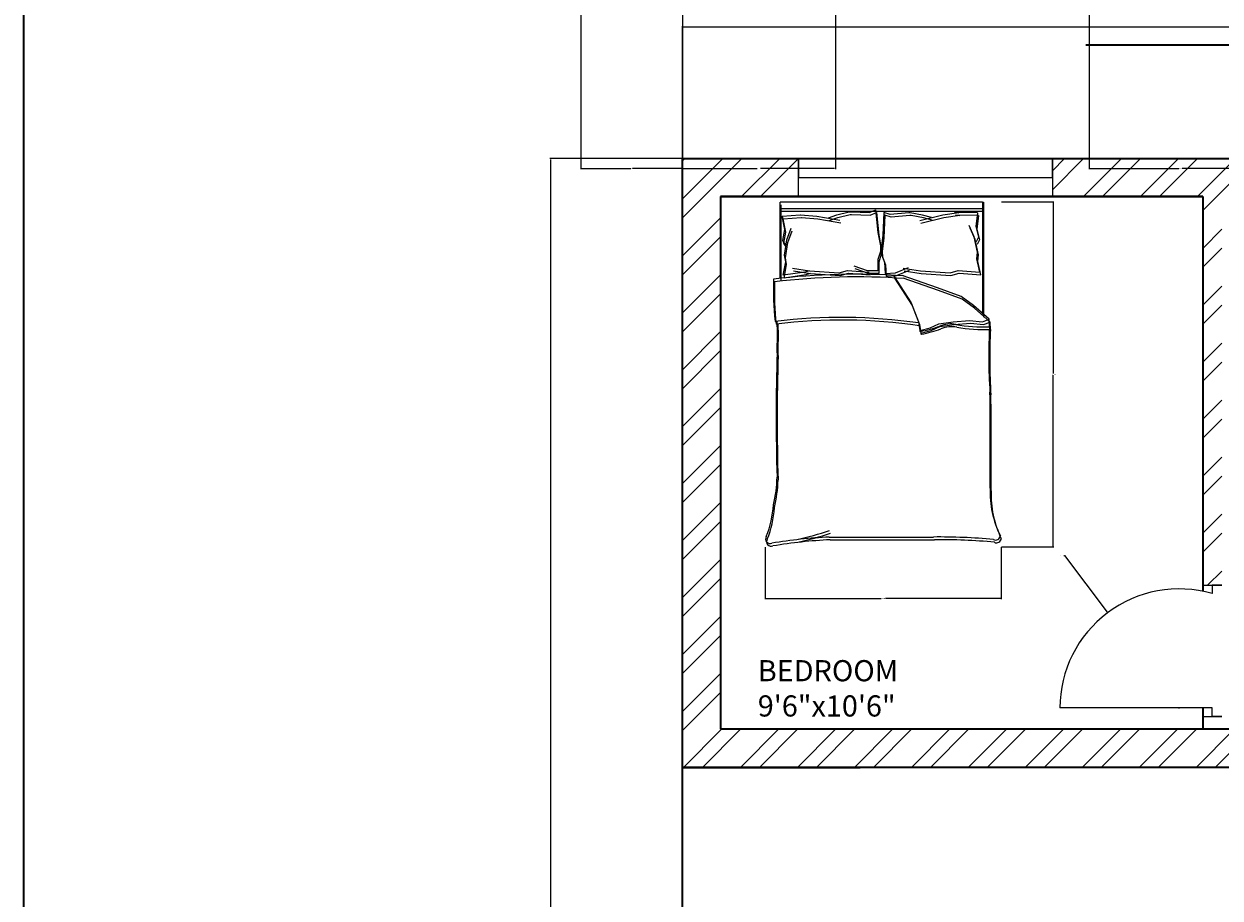
# Model space of a CAD drawing. Units: inches. Extents: x 1955 to 3324, y 980 to 3129.
# Tile 4 of 11: x 1955 to 2237, y 2282 to 2488. Entities that reach past the tile are written whole.
import ezdxf

# ---------------------------------------------------------------- set-up
doc = ezdxf.new("R2010")
doc.units = ezdxf.units.IN
for name, color, linetype, lineweight in [('A-ANNO-DIMS', 2, 'Continuous', 18), ('A-ANNO-TITL', 7, 'Continuous', 35), ('A-ANNO-TTLB', 7, 'Continuous', 35), ('A-AREA-IDEN', 7, 'Continuous', 18), ('A-DOOR', 3, 'Continuous', 18), ('A-FURN', 8, 'Continuous', 18), ('A-GLAZ', 4, 'Continuous', 18), ('A-WALL', 7, 'Continuous', 35), ('A-WALL-PATT', 252, 'Continuous', 13)]:
    doc.layers.add(name, color=color, linetype=linetype, lineweight=lineweight)
doc.styles.get("Standard").update_dxf_attribs({"font": 'arial.ttf'})
doc.dimstyles.get("Standard").update_dxf_attribs({"dimtxt": 0.18, "dimasz": 0.18, "dimexe": 0.18, "dimexo": 0.0625, "dimgap": 0.09, "dimtad": 0, "dimtih": 1, "dimtoh": 1, "dimdec": 4, "dimzin": 0, "dimdsep": 46, "dimtxsty": 'Standard', "dimcen": 0.09, "dimadec": 0, "dimazin": 0, "dimtfac": 1, "dimtdec": 4, "dimtofl": 0, "dimtmove": 0, "dimatfit": 3, "dimfxl": 1, "dimtolj": 1, "dimtzin": 0, "dimarcsym": 0})

# ---------------------------------------------------------------- blocks, each defined once
blk = doc.blocks.new('BED-WITH-PILLOWS')
for p, q in [((3.48, 63.33), (3.48, 81.44)), ((3.48, 63.33), (3.48, 81.44)), ((51.27, 81.44), (3.48, 81.44)), ((3.48, 79.91), (51.27, 79.91)), ((3.48, 79.91), (51.27, 79.91)), ((3.7, 62.69), (3.7, 80.8)), ((3.7, 62.69), (3.7, 80.8)), ((3.7, 79.27), (51.49, 79.27)), ((3.7, 79.27), (51.49, 79.27)), ((24.54, 78.99), (25.98, 79.57)), ((24.54, 78.99), (25.98, 79.57)), ((25.98, 79.57), (26.56, 74.22)), ((25.98, 79.57), (26.56, 74.22)), ((51.27, 81.44), (51.27, 54.83)), ((51.27, 81.44), (51.27, 54.83)), ((51.27, 81.44), (51.49, 81.44)), ((51.49, 81.44), (51.49, 80.8)), ((51.49, 80.8), (51.49, 54.19)), ((51.49, 80.8), (51.49, 54.19)), ((3.89, 78.13), (4.47, 74.95)), ((3.9, 78.11), (8.18, 78.43)), ((3.9, 78.11), (8.18, 78.43)), ((3.9, 78.13), (4.47, 74.95)), ((4.12, 77.49), (4.7, 74.31)), ((4.12, 77.49), (4.7, 74.31)), ((4.13, 77.47), (8.41, 77.8)), ((4.13, 77.47), (8.41, 77.8)), ((8.18, 78.43), (8.29, 78.42)), ((8.18, 78.43), (8.29, 78.42)), ((8.29, 78.42), (12.11, 78.13)), ((8.29, 78.42), (12.11, 78.13)), ((8.41, 77.8), (8.51, 77.78)), ((8.41, 77.8), (8.51, 77.78)), ((8.51, 77.78), (12.34, 77.49)), ((8.51, 77.78), (12.34, 77.49)), ((12.11, 78.13), (17.6, 77.12)), ((12.11, 78.13), (17.6, 77.12)), ((12.34, 77.49), (17.83, 76.48)), ((12.34, 77.49), (17.83, 76.48)), ((14.86, 77.69), (16.88, 78.42)), ((14.86, 77.69), (16.88, 78.42)), ((15.08, 77.05), (17.11, 77.78)), ((15.08, 77.05), (17.11, 77.78)), ((16.88, 78.42), (19.77, 79.14)), ((16.88, 78.42), (19.77, 79.14)), ((17.11, 77.78), (20, 78.5)), ((17.11, 77.78), (20, 78.5)), ((19.77, 79.14), (20.09, 79.14)), ((19.77, 79.14), (20.09, 79.14)), ((20, 78.5), (20.32, 78.5)), ((20, 78.5), (20.32, 78.5)), ((20.09, 79.14), (24.54, 78.99)), ((20.09, 79.14), (24.54, 78.99)), ((20.32, 78.5), (24.77, 78.36)), ((20.32, 78.5), (24.77, 78.36)), ((24.77, 78.36), (26.21, 78.93)), ((24.77, 78.36), (26.21, 78.93)), ((26.21, 78.93), (26.79, 73.58)), ((26.21, 78.93), (26.79, 73.58)), ((27.98, 78.95), (27.73, 73.58)), ((27.98, 78.95), (27.73, 73.58)), ((28.21, 78.31), (27.96, 72.94)), ((28.21, 78.31), (27.96, 72.94)), ((29.46, 78.46), (27.98, 78.95)), ((29.46, 78.46), (27.98, 78.95)), ((29.68, 77.83), (28.21, 78.31)), ((29.68, 77.83), (28.21, 78.31)), ((33.88, 78.89), (29.46, 78.46)), ((33.88, 78.89), (29.46, 78.46)), ((34.11, 78.25), (29.68, 77.83)), ((34.11, 78.25), (29.68, 77.83)), ((34.21, 78.91), (33.88, 78.89)), ((34.2, 78.91), (33.88, 78.89)), ((34.43, 78.27), (34.11, 78.25)), ((34.43, 78.27), (34.11, 78.25)), ((37.14, 78.36), (34.2, 78.91)), ((37.14, 78.36), (34.21, 78.91)), ((37.36, 77.73), (34.43, 78.27)), ((37.36, 77.73), (34.43, 78.27)), ((41.91, 78.37), (36.5, 77.02)), ((41.91, 78.37), (36.5, 77.02)), ((42.14, 77.73), (36.72, 76.38)), ((42.14, 77.73), (36.72, 76.38)), ((39.2, 77.77), (37.14, 78.36)), ((39.2, 77.77), (37.14, 78.36)), ((39.43, 77.13), (37.36, 77.73)), ((39.43, 77.13), (37.36, 77.73)), ((45.71, 78.9), (41.91, 78.37)), ((45.71, 78.9), (41.91, 78.37)), ((45.94, 78.26), (42.14, 77.73)), ((45.94, 78.26), (42.14, 77.73)), ((50.11, 78.89), (44.71, 78.98)), ((44.71, 78.98), (45.71, 78.9)), ((50.11, 78.89), (44.71, 78.98)), ((44.71, 78.98), (45.71, 78.9)), ((50.34, 78.25), (44.94, 78.34)), ((44.94, 78.34), (45.94, 78.26)), ((50.34, 78.25), (44.94, 78.34)), ((44.94, 78.34), (45.94, 78.26)), ((50.11, 78.89), (49.73, 75.68)), ((50.11, 78.89), (49.73, 75.68)), ((50.34, 78.25), (49.96, 75.04)), ((50.34, 78.25), (49.96, 75.04)), ((4.47, 74.95), (4.04, 72.34)), ((4.47, 74.95), (4.04, 72.34)), ((4.7, 74.31), (4.27, 71.7)), ((4.7, 74.31), (4.27, 71.7)), ((5.05, 72.49), (6.06, 75.24)), ((5.05, 72.49), (6.06, 75.24)), ((5.28, 71.85), (6.29, 74.6)), ((5.28, 71.85), (6.29, 74.6)), ((26.56, 74.22), (27.14, 71.04)), ((26.56, 74.22), (27.14, 71.04)), ((26.79, 73.58), (27.37, 70.4)), ((26.79, 73.58), (27.37, 70.4)), ((27.73, 73.58), (27.36, 70.37)), ((27.73, 73.58), (27.36, 70.37)), ((49.31, 73.19), (48.13, 75.86)), ((49.31, 73.19), (48.13, 75.86)), ((49.54, 72.55), (48.36, 75.23)), ((49.54, 72.55), (48.36, 75.23)), ((49.73, 75.68), (50.33, 73.11)), ((49.73, 75.68), (50.33, 73.11)), ((49.96, 75.04), (50.56, 72.47)), ((49.96, 75.04), (50.56, 72.47)), ((4.04, 72.34), (4.62, 71.33)), ((4.04, 72.34), (4.62, 71.33)), ((4.27, 71.7), (4.85, 70.69)), ((4.27, 71.7), (4.85, 70.69)), ((4.47, 68.87), (5.05, 72.49)), ((4.47, 68.87), (5.05, 72.49)), ((4.7, 68.23), (5.28, 71.85)), ((4.7, 68.23), (5.28, 71.85)), ((27.14, 71.04), (27.14, 69.74)), ((27.14, 71.04), (27.14, 69.74)), ((27.96, 72.94), (27.58, 69.73)), ((27.96, 72.94), (27.58, 69.73)), ((50.11, 69.61), (49.31, 73.19)), ((50.11, 69.61), (49.31, 73.19)), ((50.34, 68.98), (49.54, 72.55)), ((50.34, 68.98), (49.54, 72.55)), ((50.33, 73.11), (49.81, 72.06)), ((50.33, 73.11), (49.82, 72.06)), ((50.56, 72.47), (50.04, 71.42)), ((50.56, 72.47), (50.04, 71.42)), ((4.76, 67.28), (4.47, 68.87)), ((4.76, 67.28), (4.47, 68.87)), ((4.99, 66.64), (4.7, 68.23)), ((4.99, 66.64), (4.7, 68.23)), ((27.14, 69.74), (26.56, 67.86)), ((27.14, 69.74), (26.56, 67.86)), ((27.37, 69.1), (26.79, 67.22)), ((27.37, 69.1), (26.79, 67.22)), ((27.36, 70.37), (27.44, 69.07)), ((27.36, 70.37), (27.44, 69.07)), ((27.37, 70.4), (27.37, 69.1)), ((27.37, 70.4), (27.37, 69.1)), ((27.44, 69.07), (28.13, 67.23)), ((27.44, 69.07), (28.13, 67.23)), ((27.58, 69.73), (27.66, 68.43)), ((27.58, 69.73), (27.66, 68.43)), ((27.66, 68.43), (28.36, 66.59)), ((27.66, 68.43), (28.36, 66.59)), ((49.92, 68.01), (50.11, 69.61)), ((49.92, 68.01), (50.11, 69.61)), ((50.7, 64.87), (49.92, 68.01)), ((50.7, 64.87), (49.92, 68.01)), ((50.15, 67.37), (50.34, 68.98)), ((50.15, 67.37), (50.34, 68.98)), ((4.18, 64.1), (4.76, 67.28)), ((4.18, 64.1), (4.76, 67.28)), ((4.41, 63.46), (4.99, 66.64)), ((4.41, 63.46), (4.99, 66.64)), ((6.38, 65.81), (10.41, 65.15)), ((6.38, 65.81), (10.41, 65.15)), ((6.61, 65.18), (10.64, 64.51)), ((6.61, 65.18), (10.64, 64.51)), ((10.41, 65.15), (9.28, 64.83)), ((10.41, 65.15), (9.28, 64.83)), ((10.41, 65.15), (17.42, 64.72)), ((10.41, 65.15), (17.42, 64.72)), ((17.42, 64.72), (19.38, 65.27)), ((17.42, 64.72), (19.38, 65.27)), ((19.38, 65.27), (24.52, 64.87)), ((19.38, 65.27), (24.52, 64.87)), ((24.1, 65.18), (20.96, 66.27)), ((24.1, 65.18), (20.96, 66.27)), ((24.33, 64.54), (21.19, 65.63)), ((24.33, 64.54), (21.19, 65.63)), ((26.56, 65.18), (24.1, 65.18)), ((26.56, 65.18), (24.1, 65.18)), ((26.56, 67.86), (26.56, 65.18)), ((26.56, 67.86), (26.56, 65.18)), ((26.79, 67.22), (26.79, 64.54)), ((26.79, 67.22), (26.79, 64.54)), ((28.13, 67.23), (28.3, 64.55)), ((28.13, 67.23), (28.3, 64.55)), ((28.36, 66.59), (28.53, 63.91)), ((28.36, 66.59), (28.53, 63.91)), ((30.75, 64.7), (33.82, 65.99)), ((30.75, 64.7), (33.82, 65.99)), ((30.98, 64.06), (34.05, 65.35)), ((30.98, 64.06), (34.05, 65.35)), ((32.56, 65.81), (36.6, 65.15)), ((32.56, 65.81), (36.6, 65.15)), ((32.79, 65.18), (36.83, 64.51)), ((32.79, 65.18), (36.82, 64.51)), ((36.6, 65.15), (43.61, 64.72)), ((36.6, 65.15), (43.61, 64.72)), ((43.61, 64.72), (45.57, 65.27)), ((43.61, 64.72), (45.57, 65.27)), ((45.57, 65.27), (50.7, 64.87)), ((45.57, 65.27), (50.7, 64.87)), ((50.93, 64.23), (50.15, 67.37)), ((50.93, 64.23), (50.15, 67.37)), ((9.28, 64.83), (4.18, 64.1)), ((9.28, 64.83), (4.18, 64.1)), ((9.51, 64.19), (4.41, 63.46)), ((9.51, 64.19), (4.41, 63.46)), ((10.64, 64.51), (9.51, 64.19)), ((10.64, 64.51), (9.51, 64.19)), ((10.64, 64.51), (17.65, 64.08)), ((10.64, 64.51), (17.65, 64.08)), ((17.65, 64.08), (19.61, 64.63)), ((17.65, 64.08), (19.61, 64.63)), ((19.61, 64.63), (24.74, 64.23)), ((19.61, 64.63), (24.74, 64.23)), ((26.79, 64.54), (24.33, 64.54)), ((26.79, 64.54), (24.33, 64.54)), ((28.3, 64.55), (30.75, 64.7)), ((28.3, 64.55), (30.75, 64.7)), ((28.53, 63.91), (30.98, 64.06)), ((28.53, 63.91), (30.98, 64.06)), ((30.26, 64.06), (34.45, 57.57)), ((30.26, 64.06), (34.45, 57.57)), ((30.49, 63.42), (34.68, 56.93)), ((30.49, 63.42), (34.68, 56.93)), ((40.64, 61.13), (32.31, 64.06)), ((40.64, 61.13), (32.31, 64.06)), ((40.87, 60.49), (32.53, 63.42)), ((40.87, 60.49), (32.54, 63.42)), ((36.82, 64.51), (43.83, 64.08)), ((36.83, 64.51), (43.84, 64.08)), ((43.83, 64.08), (45.8, 64.63)), ((43.84, 64.08), (45.8, 64.63)), ((45.8, 64.63), (50.93, 64.23)), ((45.8, 64.63), (50.93, 64.23)), ((46.22, 59.11), (40.64, 61.13)), ((46.22, 59.11), (40.64, 61.13)), ((46.45, 58.48), (40.87, 60.49)), ((46.45, 58.48), (40.87, 60.49)), ((34.45, 57.57), (36.15, 53.08)), ((34.45, 57.57), (36.15, 53.08)), ((34.68, 56.93), (36.38, 52.44)), ((34.68, 56.93), (36.38, 52.44)), ((49.16, 56.95), (46.22, 59.11)), ((49.16, 56.95), (46.22, 59.11)), ((49.39, 56.31), (46.45, 58.48)), ((49.39, 56.31), (46.45, 58.48)), ((52.87, 53.7), (49.16, 56.95)), ((52.87, 53.7), (49.16, 56.95)), ((53.1, 53.06), (49.39, 56.31)), ((53.1, 53.06), (49.39, 56.31)), ((36.15, 53.08), (36.46, 51.07)), ((36.15, 53.08), (36.46, 51.07)), ((36.38, 52.44), (36.69, 50.43)), ((36.38, 52.44), (36.69, 50.43)), ((36.46, 51.07), (38.94, 51.69)), ((36.46, 51.07), (38.94, 51.69)), ((36.69, 50.43), (39.17, 51.05)), ((36.69, 50.43), (39.17, 51.05)), ((38.94, 51.69), (40.95, 52.61)), ((38.94, 51.69), (40.95, 52.61)), ((39.17, 51.05), (41.18, 51.97)), ((39.17, 51.05), (41.18, 51.97)), ((40.95, 52.61), (44.36, 53.08)), ((40.95, 52.61), (44.36, 53.08)), ((41.18, 51.97), (44.59, 52.44)), ((41.18, 51.97), (44.59, 52.44)), ((44.36, 53.08), (48.23, 53.39)), ((44.36, 53.08), (48.23, 53.39)), ((44.59, 52.44), (48.46, 52.75)), ((44.59, 52.44), (48.46, 52.75)), ((48.23, 53.39), (51.33, 53.08)), ((48.23, 53.39), (51.33, 53.08)), ((48.46, 52.75), (51.56, 52.44)), ((48.46, 52.75), (51.56, 52.44)), ((51.33, 53.08), (52.87, 53.7)), ((51.33, 53.08), (52.87, 53.7)), ((51.56, 52.44), (53.1, 53.06)), ((51.56, 52.44), (53.1, 53.06)), ((52.95, 51.95), (52.87, 53.7, 3.87)), ((52.95, 51.95), (52.87, 53.7, 3.87)), ((53.18, 51.31), (53.1, 53.06, 3.87)), ((53.18, 51.31), (53.1, 53.06, 3.87)), ((15.06, 2.2), (39.68, 2.2)), ((15.06, 2.2), (39.68, 2.2)), ((15.29, 1.56), (39.91, 1.56)), ((15.29, 1.56), (39.91, 1.56))]:
    blk.add_line(p, q)
for centre, radius, start, end in [((85.16, 61.35), 83.31, 178.7218, 185.604), ((85.16, 61.35), 83.31, 178.7218, 185.604), ((21.36, -100.61), 164.97, 86.0865, 96.7821), ((21.36, -100.61), 164.97, 86.0865, 96.7821), ((85.39, 60.71), 83.31, 178.7218, 185.604), ((85.39, 60.71), 83.31, 178.7218, 185.604), ((21.59, -101.25), 164.97, 86.0865, 96.7821), ((21.59, -101.25), 164.97, 86.0865, 96.7821), ((17.76, -74.87), 129.02, 81.7845, 96.9006), ((17.76, -74.87), 129.02, 81.7845, 96.9006), ((17.98, -75.51), 129.02, 81.7845, 96.9006), ((17.98, -75.51), 129.02, 81.7845, 96.9006), ((-167.31, 50.27), 170.11, 358.4762, 1.0082), ((-167.31, 50.27), 170.11, 358.4762, 1.0082), ((-167.08, 49.63), 170.11, 358.4762, 1.0082), ((-167.08, 49.63), 170.11, 358.4762, 1.0082), ((36.64, 51), 0.185, 160.2464, 271.1377), ((36.64, 51), 0.185, 160.2464, 271.1377), ((31.15, 79.96), 29.65, 280.6617, 289.8806), ((31.15, 79.96), 29.65, 280.6617, 289.8806), ((31.38, 79.32), 29.65, 280.6617, 289.8806), ((31.38, 79.32), 29.65, 280.6617, 289.8806), ((43.74, 46.38), 6.22, 78.6608, 113.7384), ((43.74, 46.38), 6.22, 78.6608, 113.7384), ((43.97, 45.74), 6.22, 78.6608, 113.7384), ((43.97, 45.74), 6.22, 78.6608, 113.7384), ((51.33, 88.1), 36.18, 259.8763, 272.5657), ((51.33, 88.1), 36.18, 259.8763, 272.5657), ((51.56, 87.46), 36.18, 259.8763, 272.5657), ((51.56, 87.46), 36.18, 259.8763, 272.5657), ((182.27, 45.13), 129.5, 176.9791, 183.8365), ((182.27, 45.13), 129.5, 176.9791, 183.8365), ((182.49, 44.49), 129.5, 176.9791, 183.8365), ((182.49, 44.49), 129.5, 176.9791, 183.8365), ((36.87, 50.36), 0.185, 160.2464, 271.1377), ((36.86, 50.36), 0.185, 160.2464, 271.1377), ((484.82, 30.83), 482.31, 178.2277, 181.7185), ((484.82, 30.83), 482.31, 178.2277, 181.7185), ((485.05, 30.19), 482.31, 178.2277, 181.7185), ((485.05, 30.19), 482.31, 178.2277, 181.7185), ((-4508.74, 13.62), 4561.86, 0.00217, 0.28689), ((-4508.74, 13.62), 4561.86, 0.00217, 0.28689), ((-4508.51, 12.98), 4561.86, 0.00217, 0.28689), ((-4508.51, 12.98), 4561.86, 0.00217, 0.28689), ((-26.9, 16.93), 29.63, 346.0648, 358.9113), ((-26.9, 16.93), 29.63, 346.0648, 358.9113), ((-26.67, 16.29), 29.63, 346.0648, 358.9113), ((-26.67, 16.29), 29.63, 346.0648, 358.9113), ((76.16, 12.78), 23.07, 177.4714, 206.4681), ((76.16, 12.78), 23.07, 177.4714, 206.4681), ((76.39, 12.14), 23.07, 177.4714, 206.4681), ((76.39, 12.14), 23.07, 177.4714, 206.4681), ((-21.66, 11.17), 23.56, 337.9751, 356.652), ((-21.66, 11.17), 23.56, 337.9751, 356.652), ((-21.43, 10.53), 23.56, 337.9751, 356.652), ((-21.43, 10.53), 23.56, 337.9751, 356.652), ((-17.22, 105.16), 106.46, 283.3832, 287.7053), ((-17.22, 105.16), 106.46, 283.3832, 287.7053), ((-16.99, 104.52), 106.46, 283.3832, 287.7053), ((-16.99, 104.52), 106.46, 283.3832, 287.7053), ((1.09, 1.73), 1.09, 146.1736, 293.4781), ((1.09, 1.73), 1.09, 146.1736, 293.4781), ((1.32, 1.09), 1.09, 146.1736, 293.4781), ((1.32, 1.09), 1.09, 146.1736, 293.4781), ((21.43, -119.39), 121.76, 92.9958, 99.4091), ((21.43, -119.39), 121.76, 92.9958, 99.4091), ((21.66, -120.03), 121.76, 92.9958, 99.4091), ((21.66, -120.03), 121.76, 92.9958, 99.4091), ((41.15, -130.83), 133.04, 84.4998, 90.6351), ((41.15, -130.83), 133.04, 84.4998, 90.6351), ((41.38, -131.47), 133.04, 84.4998, 90.6351), ((41.38, -131.47), 133.04, 84.4998, 90.6351), ((54.41, 2.57), 1.1, 242.6588, 356.02), ((54.41, 2.57), 1.1, 242.6588, 356.02), ((54.64, 1.93), 1.1, 242.6588, 356.02), ((54.64, 1.93), 1.1, 242.6588, 356.02)]:
    blk.add_arc(centre, radius, start, end)
blk = doc.blocks.new('DOOR-BED-N')
for p, q in [((33.75, 31.05), (38.25, 31.05)), ((38.25, 31.05), (36, 31.05)), ((36, 31.05), (36, 29.05)), ((36, 2), (0, 2)), ((36, 0), (36, 2)), ((33.75, 0), (38.25, 0)), ((38.25, 0), (36, 0))]:
    blk.add_line(p, q)
blk.add_arc((28.16, 2), 28.16, 73.8433, 180)
blk = doc.blocks.new('WIN-PLAN-60-B')
for p, q in [((0, 0), (0, 9)), ((0, 9), (0, 4.5)), ((60, 4.5), (60, 9)), ((60, 9), (60, 0)), ((0, 4.5), (60, 4.5))]:
    blk.add_line(p, q)
blk = doc.blocks.new('*D53')
at = {"layer": 'A-ANNO-DIMS', "color": 0, "lineweight": -2, "transparency": 16777216}
for p, q in [((2185.66, 2446.23), (2198.01, 2446.23)), ((2197.83, 2446.05), (2197.83, 2405.63)), ((2197.83, 2364.86), (2197.83, 2405.27)), ((2185.66, 2364.68), (2198.01, 2364.68))]:
    blk.add_line(p, q, dxfattribs=at)
at = {"layer": 'A-ANNO-DIMS', "color": 0, "transparency": 16777216}
for points in [[(2197.8, 2446.05), (2197.86, 2446.05), (2197.83, 2446.23)], [(2197.8, 2364.86), (2197.86, 2364.86), (2197.83, 2364.68)]]:
    blk.add_solid(points, dxfattribs=at)
at = {"layer": 'Defpoints', "color": 0, "transparency": 16777216}
for p in [(2185.6, 2446.23), (2197.83, 2446.23), (2185.6, 2364.68)]:
    blk.add_point(p, dxfattribs=at)
at = {"layer": 'A-ANNO-DIMS', "color": 0, "transparency": 16777216, "insert": (2197.83, 2405.45), "char_height": 0.18, "attachment_point": 5}
blk.add_mtext('\\A1;BED 82 TYP.', dxfattribs=at)
blk = doc.blocks.new('*D54')
at = {"layer": 'A-ANNO-DIMS', "color": 0, "lineweight": -2, "transparency": 16777216}
for p, q in [((2129.77, 2364.62), (2129.77, 2352.27)), ((2185.6, 2364.62), (2185.6, 2352.27)), ((2129.95, 2352.45), (2157.16, 2352.45)), ((2185.42, 2352.45), (2158.21, 2352.45))]:
    blk.add_line(p, q, dxfattribs=at)
at = {"layer": 'A-ANNO-DIMS', "color": 0, "transparency": 16777216}
for points in [[(2129.95, 2352.48), (2129.95, 2352.42), (2129.77, 2352.45)], [(2185.42, 2352.48), (2185.42, 2352.42), (2185.6, 2352.45)]]:
    blk.add_solid(points, dxfattribs=at)
at = {"layer": 'Defpoints', "color": 0, "transparency": 16777216}
for p in [(2129.77, 2364.68), (2185.6, 2364.68), (2185.6, 2352.45)]:
    blk.add_point(p, dxfattribs=at)
at = {"layer": 'A-ANNO-DIMS', "color": 0, "transparency": 16777216, "insert": (2157.68, 2352.45), "char_height": 0.18, "attachment_point": 5}
blk.add_mtext('\\A1;56 TYP.', dxfattribs=at)
blk = doc.blocks.new('*D91')
at = {"layer": 'A-ANNO-DIMS', "color": 0, "lineweight": -2, "transparency": 16777216}
for p, q in [((2110.21, 2456.57), (2110.21, 2487.83)), ((2110.39, 2487.65), (2312.42, 2487.65)), ((2515.03, 2487.65), (2313, 2487.65)), ((2515.21, 2456.57), (2515.21, 2487.83))]:
    blk.add_line(p, q, dxfattribs=at)
at = {"layer": 'A-ANNO-DIMS', "color": 0, "transparency": 16777216}
for points in [[(2110.39, 2487.68), (2110.39, 2487.62), (2110.21, 2487.65)], [(2515.03, 2487.68), (2515.03, 2487.62), (2515.21, 2487.65)]]:
    blk.add_solid(points, dxfattribs=at)
at = {"layer": 'Defpoints', "color": 0, "transparency": 16777216}
for p in [(2515.21, 2487.65), (2110.21, 2456.5), (2515.21, 2456.5)]:
    blk.add_point(p, dxfattribs=at)
at = {"layer": 'A-ANNO-DIMS', "color": 0, "transparency": 16777216, "insert": (2312.71, 2487.65), "char_height": 0.18, "attachment_point": 5}
blk.add_mtext('\\A1;405', dxfattribs=at)
blk = doc.blocks.new('*D92')
at = {"layer": 'A-ANNO-DIMS', "color": 0, "lineweight": -2, "transparency": 16777216}
for p, q in [((2110.15, 2456.5), (2078.88, 2456.5)), ((2079.06, 2456.32), (2079.06, 2176.69)), ((2079.06, 1896.68), (2079.06, 2176.32)), ((2110.15, 1896.5), (2078.88, 1896.5))]:
    blk.add_line(p, q, dxfattribs=at)
at = {"layer": 'A-ANNO-DIMS', "color": 0, "transparency": 16777216}
for points in [[(2079.03, 2456.32), (2079.09, 2456.32), (2079.06, 2456.5)], [(2079.03, 1896.68), (2079.09, 1896.68), (2079.06, 1896.5)]]:
    blk.add_solid(points, dxfattribs=at)
at = {"layer": 'Defpoints', "color": 0, "transparency": 16777216}
for p in [(2079.06, 2456.5), (2110.21, 2456.5), (2110.21, 1896.5)]:
    blk.add_point(p, dxfattribs=at)
at = {"layer": 'A-ANNO-DIMS', "color": 0, "transparency": 16777216, "insert": (2079.06, 2176.5), "char_height": 0.18, "attachment_point": 5}
blk.add_mtext('\\A1;560', dxfattribs=at)
blk = doc.blocks.new('*D114')
at = {"layer": 'A-ANNO-DIMS', "color": 0, "lineweight": -2, "transparency": 16777216}
for p, q in [((2110.21, 2616.69), (2110.21, 2454)), ((2086.21, 2610.35), (2086.21, 2454)), ((2086.39, 2454.18), (2097.99, 2454.18)), ((2110.03, 2454.18), (2098.43, 2454.18))]:
    blk.add_line(p, q, dxfattribs=at)
at = {"layer": 'A-ANNO-DIMS', "color": 0, "transparency": 16777216}
for points in [[(2086.39, 2454.21), (2086.39, 2454.15), (2086.21, 2454.18)], [(2110.03, 2454.21), (2110.03, 2454.15), (2110.21, 2454.18)]]:
    blk.add_solid(points, dxfattribs=at)
at = {"layer": 'Defpoints', "color": 0, "transparency": 16777216}
for p in [(2110.21, 2616.75), (2086.21, 2610.41), (2110.21, 2454.18)]:
    blk.add_point(p, dxfattribs=at)
at = {"layer": 'A-ANNO-DIMS', "color": 0, "transparency": 16777216, "insert": (2098.21, 2454.18), "char_height": 0.18, "attachment_point": 5}
blk.add_mtext('\\A1;24', dxfattribs=at)
blk = doc.blocks.new('*D115')
at = {"layer": 'A-ANNO-DIMS', "color": 0, "lineweight": -2, "transparency": 16777216}
for p, q in [((2110.21, 2610.35), (2110.21, 2454)), ((2146.36, 2610.35), (2146.36, 2454)), ((2110.39, 2454.18), (2127.89, 2454.18)), ((2146.18, 2454.18), (2128.68, 2454.18))]:
    blk.add_line(p, q, dxfattribs=at)
at = {"layer": 'A-ANNO-DIMS', "color": 0, "transparency": 16777216}
for points in [[(2110.39, 2454.21), (2110.39, 2454.15), (2110.21, 2454.18)], [(2146.18, 2454.21), (2146.18, 2454.15), (2146.36, 2454.18)]]:
    blk.add_solid(points, dxfattribs=at)
at = {"layer": 'Defpoints', "color": 0, "transparency": 16777216}
for p in [(2110.21, 2610.41), (2146.36, 2610.41), (2146.36, 2454.18)]:
    blk.add_point(p, dxfattribs=at)
at = {"layer": 'A-ANNO-DIMS', "color": 0, "transparency": 16777216, "insert": (2128.29, 2454.18), "char_height": 0.18, "attachment_point": 5}
blk.add_mtext('\\A1;36.15', dxfattribs=at)
blk = doc.blocks.new('*D116')
at = {"layer": 'A-ANNO-DIMS', "color": 0, "lineweight": -2, "transparency": 16777216}
for p, q in [((2206.36, 2610.35), (2206.36, 2454)), ((2249.49, 2610.35), (2249.49, 2454)), ((2206.54, 2454.18), (2227.53, 2454.18)), ((2249.31, 2454.18), (2228.32, 2454.18))]:
    blk.add_line(p, q, dxfattribs=at)
at = {"layer": 'A-ANNO-DIMS', "color": 0, "transparency": 16777216}
for points in [[(2206.54, 2454.21), (2206.54, 2454.15), (2206.36, 2454.18)], [(2249.31, 2454.21), (2249.31, 2454.15), (2249.49, 2454.18)]]:
    blk.add_solid(points, dxfattribs=at)
at = {"layer": 'Defpoints', "color": 0, "transparency": 16777216}
for p in [(2206.36, 2610.41), (2249.49, 2610.41), (2249.49, 2454.18)]:
    blk.add_point(p, dxfattribs=at)
at = {"layer": 'A-ANNO-DIMS', "color": 0, "transparency": 16777216, "insert": (2227.93, 2454.18), "char_height": 0.18, "attachment_point": 5}
blk.add_mtext('\\A1;43.13', dxfattribs=at)
blk = doc.blocks.new('*D141')
at = {"layer": 'A-ANNO-DIMS', "color": 0, "lineweight": -2, "transparency": 16777216}
for p, q in [((2200.37, 2362.58), (2200.55, 2362.58)), ((2200.55, 2362.58), (2210.6, 2349.21)), ((2227.53, 2326.55), (2227.71, 2326.55)), ((2227.62, 2326.46), (2227.62, 2326.64))]:
    blk.add_line(p, q, dxfattribs=at)
at = {"layer": 'A-ANNO-DIMS', "color": 0, "transparency": 16777216}
blk.add_solid([(2210.62, 2349.23), (2210.57, 2349.19), (2210.71, 2349.07)], dxfattribs=at)
at = {"layer": 'Defpoints', "color": 0, "transparency": 16777216}
for p in [(2210.71, 2349.07), (2227.62, 2326.55)]:
    blk.add_point(p, dxfattribs=at)
at = {"layer": 'A-ANNO-DIMS', "color": 0, "transparency": 16777216, "insert": (2199.82, 2362.58), "char_height": 0.18, "attachment_point": 5}
blk.add_mtext('\\A1;R28.163', dxfattribs=at)

msp = doc.modelspace()

# ---------------------------------------------------------------- hatches: boundary and pattern name
at = {"layer": 'A-WALL-PATT'}
h = msp.add_hatch(dxfattribs=at)
h.set_pattern_fill('ANSI32', color=256)
h.paths.add_polyline_path([(2361.4775, 2456.5037), (2270.2755, 2456.5037), (2270.2755, 2447.5037), (2285.7102, 2447.5037), (2285.7102, 2363.5037), (2281.1795, 2363.5037), (2281.1795, 2359.0037), (2290.2102, 2359.0037), (2290.2102, 2447.5037), (2361.4775, 2447.5037), (2361.4775, 2452.0037)])
h.paths.add_polyline_path([(2246.2755, 2456.5037), (2197.6809, 2456.5037), (2197.6809, 2447.5037), (2233.2102, 2447.5037), (2233.2102, 2355.6044), (2237.7102, 2355.6044), (2237.7102, 2447.5037), (2246.2755, 2447.5037)], flags=17)
h.paths.add_polyline_path([(2137.6809, 2456.5037), (2110.2102, 2456.5037), (2110.2102, 2312.5037), (2152.2102, 2312.5037), (2281.2102, 2312.5037), (2281.2102, 2107.6185), (2290.2102, 2107.6185), (2290.2102, 2267.9289), (2329.216, 2267.9289), (2329.216, 2272.4289), (2329.216, 2276.9289), (2290.2102, 2276.9289), (2290.2102, 2321.5037), (2281.2102, 2321.5037), (2119.2102, 2321.5037), (2119.2102, 2447.5037), (2137.6809, 2447.5037)])
h.paths.add_polyline_path([(2515.2102, 2456.5037), (2421.4775, 2456.5037), (2421.4775, 2447.5037), (2506.2102, 2447.5037), (2506.2102, 2415.6626), (2515.2102, 2415.6626)])
h.paths.add_polyline_path([(2515.2102, 2355.6626), (2506.2102, 2355.6626), (2506.2102, 2321.5037), (2424.9282, 2321.5037), (2424.9282, 2312.5037), (2461.2102, 2312.5037), (2470.2102, 2312.5037), (2515.2102, 2312.5037)])
h.paths.add_polyline_path([(2515.2102, 2232.5037), (2470.2102, 2232.5037), (2470.2102, 2237.3759), (2465.7102, 2237.3759), (2461.2102, 2237.3759), (2461.2102, 2232.5037), (2377.2219, 2232.5037), (2377.2219, 2321.5037), (2368.2219, 2321.5037), (2368.2219, 2276.9289), (2359.3802, 2276.9289), (2359.3802, 2272.4289), (2359.3802, 2267.9289), (2368.2219, 2267.9289), (2368.2219, 2223.5037), (2377.2219, 2223.5037), (2461.2102, 2223.5037), (2506.2102, 2223.5037), (2506.2102, 2129.5037), (2461.2102, 2129.5037), (2387.2102, 2129.5037), (2368.2219, 2129.5037), (2368.2219, 2056.4936), (2361.0095, 2056.4936), (2361.0095, 2051.9936), (2361.0095, 2047.4936), (2368.2219, 2047.4936), (2368.2219, 2031.5037), (2377.2219, 2031.5037), (2377.2219, 2120.5037), (2461.2102, 2120.5037), (2461.2102, 2112.7921), (2470.2102, 2112.7921), (2470.2102, 2120.5037), (2515.2102, 2120.5037), (2515.2102, 2129.5037)])
h.paths.add_polyline_path([(2470.2102, 2277.1758), (2461.2102, 2277.1758), (2461.2102, 2272.5037), (2461.2102, 2270.2549), (2470.2102, 2270.2549), (2470.2102, 2272.5037)], flags=17)
h.paths.add_polyline_path([(2515.2102, 2040.5037), (2470.2102, 2040.5037), (2417.8264, 2040.5037), (2417.8264, 2031.5037), (2506.2102, 2031.5037), (2506.2102, 2005.3639), (2515.2102, 2005.3639)])
h.paths.add_polyline_path([(2506.2102, 1905.5037), (2402.6963, 1905.5037), (2402.6963, 1896.5037), (2506.2102, 1896.5037)])
h.paths.add_polyline_path([(2515.2102, 1945.3639), (2506.2102, 1945.3639), (2506.2102, 1905.5037), (2506.2102, 1896.5037), (2515.2102, 1896.5037)])
h.paths.add_polyline_path([(2342.6963, 1901.0037), (2342.6963, 1905.5037), (2273.4892, 1905.5037), (2273.4892, 1896.5037), (2342.6963, 1896.5037)])
h.paths.add_polyline_path([(2290.2102, 1994.0037), (2283.612, 1994.0037), (2283.612, 1991.7537), (2283.612, 1989.5037), (2285.7102, 1989.5037), (2285.7102, 1905.5037), (2290.2102, 1905.5037)])
h.paths.add_polyline_path([(2249.4892, 1905.5037), (2237.7102, 1905.5037), (2206.3617, 1905.5037), (2206.3617, 1896.5037), (2249.4892, 1896.5037), (2249.4892, 1901.0037)])
h.paths.add_polyline_path([(2237.7102, 1989.5037), (2261.7102, 1989.5037), (2261.7102, 1994.0037), (2237.7102, 1994.0037), (2237.7102, 1999.266), (2235.4602, 1999.266), (2233.2102, 1999.266), (2233.2102, 1994.0037), (2233.2102, 1905.5037), (2237.7102, 1905.5037)])
h.paths.add_polyline_path([(2119.2102, 1947.5144), (2110.2102, 1947.5144), (2110.2102, 1896.5037), (2119.2102, 1896.5037), (2146.3617, 1896.5037), (2146.3617, 1901.0037), (2146.3617, 1905.5037), (2119.2102, 1905.5037)])
h.paths.add_polyline_path([(2119.2102, 2068.6379), (2110.2102, 2068.6379), (2110.2102, 2007.5144), (2119.2102, 2007.5144), (2119.2102, 2031.5037), (2233.2102, 2031.5037), (2233.2102, 2027.9287), (2235.4602, 2027.9287), (2237.7102, 2027.9287), (2237.7102, 2031.5037), (2281.2102, 2031.5037), (2290.2102, 2031.5037), (2290.2102, 2047.4936), (2326.409, 2047.4936), (2326.409, 2056.4936), (2290.2102, 2056.4936), (2290.2102, 2071.2722), (2285.7102, 2071.2722), (2281.2102, 2071.2722), (2281.2102, 2040.5037), (2227.2102, 2040.5037), (2227.2102, 2111.2571), (2222.7102, 2111.2571), (2218.2102, 2111.2571), (2218.2102, 2040.5037), (2119.2102, 2040.5037)])
h.paths.add_polyline_path([(2236.9166, 2214.5037), (2161.2102, 2214.5037), (2161.2102, 2221.6488), (2152.2102, 2221.6488), (2152.2102, 2214.5037), (2110.2102, 2214.5037), (2110.2102, 2205.5037), (2131.2394, 2205.5037), (2131.2394, 2198.3478), (2140.2394, 2198.3478), (2140.2394, 2205.5037), (2224.2394, 2205.5037), (2224.2394, 2200.2317), (2228.7394, 2200.2317), (2233.2394, 2200.2317), (2233.2394, 2205.5037), (2236.9166, 2205.5037)], flags=17)
h.paths.add_polyline_path([(2236.9166, 2157.5037), (2233.2394, 2157.5037), (2233.2394, 2178.9172), (2228.7394, 2178.9172), (2224.2394, 2178.9172), (2224.2394, 2157.5037), (2140.2394, 2157.5037), (2140.2394, 2174.3478), (2131.2394, 2174.3478), (2131.2394, 2157.5037), (2110.2102, 2157.5037), (2110.2102, 2128.6379), (2119.2102, 2128.6379), (2119.2102, 2148.5037), (2218.2102, 2148.5037), (2218.2102, 2141.7262), (2222.7102, 2141.7262), (2227.2102, 2141.7262), (2227.2102, 2148.5037), (2236.9166, 2148.5037)], flags=0)
h.paths.add_polyline_path([(3084.7449, 2537.3808), (3212.7954, 2537.3808), (3212.7954, 2555.9271), (3084.7449, 2555.9271)], flags=9)
h.paths.add_polyline_path([(3068.7485, 2853.43), (3169.977, 2853.43), (3169.977, 2871.9764), (3068.7485, 2871.9764)], flags=9)
h.paths.add_polyline_path([(3074.1798, 2918.0252), (3126.4732, 2918.0252), (3126.4732, 2936.5716), (3074.1798, 2936.5716)], flags=9)
h.paths.add_polyline_path([(3073.0928, 2947.3127), (3199.0499, 2947.3127), (3199.0499, 2965.8591), (3073.0928, 2965.8591)], flags=9)
h.paths.add_polyline_path([(2733.8393, 2484.8678), (2879.7915, 2484.8678), (2879.7915, 2521.9606), (2733.8393, 2521.9606)], flags=9)
h.paths.add_polyline_path([(2204.9881, 2482.4168), (2355.1272, 2482.4168), (2355.1272, 2519.5095), (2204.9881, 2519.5095)], flags=9)
h.paths.add_polyline_path([(3062.1429, 2387.2466), (3079.3735, 2387.2466), (3079.3735, 2411.9751), (3062.1429, 2411.9751)], flags=9)
h.paths.add_polyline_path([(2190.1574, 2158.8439), (2219.315, 2158.8439), (2219.315, 2177.5013), (2190.1574, 2177.5013)], flags=25)
h.paths.add_polyline_path([(2213.6766, 1840.7276), (2405.0382, 1840.7276), (2405.0382, 1865.4561), (2213.6766, 1865.4561)], flags=9)
h.paths.add_polyline_path([(2180.5398, 2233.911), (2213.9471, 2233.911), (2213.9471, 2252.5683), (2180.5398, 2252.5683)], flags=25)
h.paths.add_polyline_path([(2134.4484, 2238.3973), (2134.4484, 2274.2807), (2115.791, 2274.2807), (2115.791, 2238.3973)], flags=25)
h.paths.add_polyline_path([(2135.1593, 2122.9991), (2173.7507, 2122.9991), (2173.7507, 2141.6565), (2135.1593, 2141.6565)], flags=25)
h.paths.add_polyline_path([(2129.8822, 2002.1912), (2168.4736, 2002.1912), (2168.4736, 2020.8486), (2129.8822, 2020.8486)], flags=9)
h.paths.add_polyline_path([(2239.6647, 1953.4107), (2268.8973, 1953.4107), (2268.8973, 1972.068), (2239.6647, 1972.068)], flags=9)
h.paths.add_polyline_path([(2352.8562, 1951.2904), (2402.1775, 1951.2904), (2402.1775, 1969.9477), (2352.8562, 1969.9477)], flags=9)
h.paths.add_polyline_path([(2500.1358, 2055.32), (2500.1358, 2091.2034), (2481.4784, 2091.2034), (2481.4784, 2055.32)], flags=25)
h.paths.add_polyline_path([(2391.2702, 2058.6821), (2424.4285, 2058.6821), (2424.4285, 2077.3394), (2391.2702, 2077.3394)], flags=25)
h.paths.add_polyline_path([(2507.7996, 2257.2758), (2507.7996, 2293.1592), (2489.1422, 2293.1592), (2489.1422, 2257.2758)], flags=25)
h.paths.add_polyline_path([(2386.8349, 2273.8734), (2419.9931, 2273.8734), (2419.9931, 2292.5307), (2386.8349, 2292.5307)], flags=25)
h.paths.add_polyline_path([(2335.374, 2373.3267), (2384.6953, 2373.3267), (2384.6953, 2391.984), (2335.374, 2391.984)], flags=9)
h.paths.add_polyline_path([(2243.8205, 2380.6539), (2273.0531, 2380.6539), (2273.0531, 2399.3113), (2243.8205, 2399.3113)], flags=25)
h.paths.add_polyline_path([(2126.2627, 2321.6894), (2164.8541, 2321.6894), (2164.8541, 2340.3467), (2126.2627, 2340.3467)], flags=25)

# ---------------------------------------------------------------- linework, layer by layer
at = {"layer": 'A-ANNO-TITL'}
msp.add_line((2205.5822, 2483.435), (2353.4472, 2483.435), dxfattribs=at)
at = {"layer": 'A-ANNO-TTLB'}
msp.add_lwpolyline([(1954.5391, 3128.9103), (3323.9705, 3128.9103), (3323.9705, 1703.6826), (1954.5391, 1703.6826)], close=True, dxfattribs=at)
at = {"layer": 'A-WALL'}
for p, q in [((2110.2102, 2456.5037), (2515.2102, 2456.5037)), ((2110.2102, 1896.5037), (2110.2102, 2456.5037)), ((2119.2102, 2447.5037), (2233.2102, 2447.5037)), ((2233.2102, 2447.5037), (2119.2102, 2447.5037)), ((2119.2102, 2447.5037), (2119.2102, 2321.5037)), ((2233.2102, 2447.5037), (2233.2102, 2354.157)), ((2233.2102, 2326.5535), (2233.2102, 2321.5037)), ((2290.2102, 2321.5037), (2119.2102, 2321.5037)), ((2281.2102, 2312.5037), (2110.2102, 2312.5037)), ((2110.2102, 2312.5037), (2152.2102, 2312.5037))]:
    msp.add_line(p, q, dxfattribs=at)

# ---------------------------------------------------------------- block references
at = {"layer": 'A-DOOR'}
msp.add_blockref('DOOR-BED-N', (2199.46, 2324.554), dxfattribs=at)
at = {"layer": 'A-FURN'}
msp.add_blockref('BED-WITH-PILLOWS', (2129.858, 2364.784), dxfattribs=at)
at = {"layer": 'A-GLAZ'}
msp.add_blockref('WIN-PLAN-60-B', (2137.681, 2447.504), dxfattribs=at)

# ---------------------------------------------------------------- texts
at = {"layer": 'A-AREA-IDEN', "insert": (2128.0243, 2337.8621), "char_height": 5, "attachment_point": 1}
msp.add_mtext_dynamic_manual_height_columns('BEDROOM\\P9\'6"x10\'6"', width=107.165227, gutter_width=12.5, heights=[0], dxfattribs=at)

# ---------------------------------------------------------------- dimensions: what is measured, and where the dimension line sits
at = {"layer": 'A-ANNO-DIMS'}
for base, p1, p2, override, picture, middle in [((2110.2102, 2454.185), (2086.2102, 2610.4103), (2110.2102, 2616.7505), {"dimdec": 0, "dimlfac": 1, "dimrnd": 0, "dimzin": 0, "dimdsep": 46, "dimlunit": 2}, '*D114', (2098.2102, 2454.185)), ((2146.3617, 2454.185), (2110.2102, 2610.4103), (2146.3617, 2610.4103), {"dimdec": 2, "dimlfac": 1, "dimrnd": 0, "dimzin": 0, "dimdsep": 46, "dimlunit": 2}, '*D115', (2128.286, 2454.185)), ((2249.4892, 2454.185), (2206.3617, 2610.4103), (2249.4892, 2610.4103), {"dimdec": 2, "dimlfac": 1, "dimrnd": 0, "dimzin": 0, "dimdsep": 46, "dimlunit": 2}, '*D116', (2227.9254, 2454.185)), ((2515.2102, 2487.6537), (2110.2102, 2456.5037), (2515.2102, 2456.5037), {"dimdec": 0, "dimlfac": 1, "dimrnd": 0, "dimzin": 0, "dimdsep": 46, "dimlunit": 2}, '*D91', (2312.7102, 2487.6537))]:
    dim = msp.add_linear_dim(base=base, p1=p1, p2=p2, dimstyle='Standard', override=override, dxfattribs=at)
    dim.commit()
    dim.dimension.update_dxf_attribs({"geometry": picture, "text_midpoint": middle})
dim = msp.add_linear_dim(base=(2079.0602, 2456.5037), p1=(2110.2102, 1896.5037), p2=(2110.2102, 2456.5037), angle=90, dimstyle='Standard', override={"dimdec": 0, "dimlfac": 1, "dimrnd": 0, "dimzin": 0, "dimdsep": 46, "dimlunit": 2}, dxfattribs=at)
dim.commit()
dim.dimension.update_dxf_attribs({"geometry": '*D92', "text_midpoint": (2079.0602, 2176.5037)})
dim = msp.add_linear_dim(base=(2197.8288, 2446.2274), p1=(2185.5965, 2364.6787), p2=(2185.5965, 2446.2274), angle=90, text='BED <> TYP.', dimstyle='Standard', override={"dimdec": 0, "dimlfac": 1, "dimrnd": 0, "dimzin": 0, "dimdsep": 46, "dimlunit": 2}, dxfattribs=at)
dim.commit()
dim.dimension.update_dxf_attribs({"geometry": '*D53', "text_midpoint": (2197.8288, 2405.453)})
dim = msp.add_linear_dim(base=(2185.5965, 2352.4464), p1=(2129.772, 2364.6787), p2=(2185.5965, 2364.6787), text='<> TYP.', dimstyle='Standard', override={"dimdec": 0, "dimlfac": 1, "dimrnd": 0, "dimzin": 0, "dimdsep": 46, "dimlunit": 2}, dxfattribs=at)
dim.commit()
dim.dimension.update_dxf_attribs({"geometry": '*D54', "text_midpoint": (2157.6843, 2352.4464)})
dim = msp.add_radius_dim(center=(2227.6234, 2326.5535), mpoint=(2210.7052, 2349.0688), dimstyle='Standard', override={"dimdec": 3, "dimlfac": 1, "dimrnd": 0, "dimzin": 0, "dimdsep": 46, "dimlunit": 2}, dxfattribs=at)
dim.commit()
dim.dimension.update_dxf_attribs({"geometry": '*D141', "text_midpoint": (2199.8244, 2362.578), "dimtype": 164})

doc.saveas('drawing.dxf')
